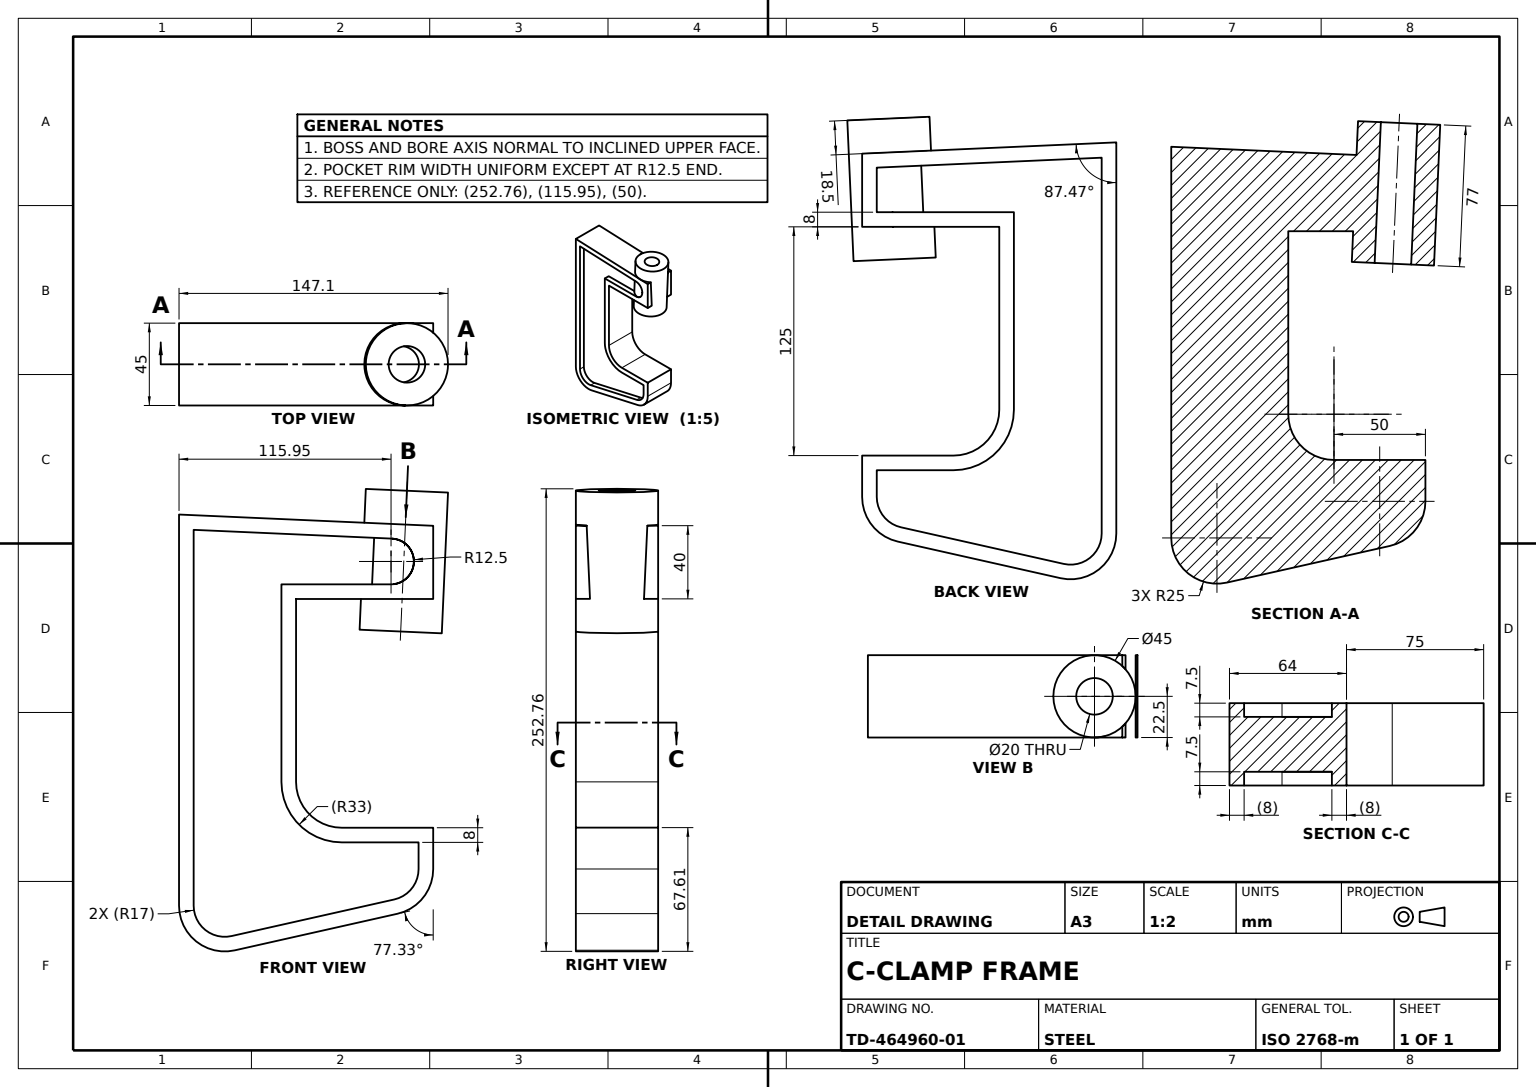
SolidWorks part; units mm, degrees
material "Plain Carbon Steel"
ref_plane "Front Plane" through (0, 0, 0) normal (0, 0, 1) x (1, 0, 0)
ref_plane "Top Plane" through (0, 0, 0) normal (0, 1, 0) x (1, 0, 0)
ref_plane "Right Plane" through (0, 0, 0) normal (1, 0, 0) x (0, 0, -1)
sketch "C Frame Profile Sketch" plane through (0, 0, 0) normal (0, 0, 1) x (1, 0, 0)
  line L0 (108.5187, 232) -> (-30.4813, 238.1503)
  line L1 (-30.4813, 238.1503) -> (-30.4813, 24.3917)
  line L2 (0, 0) -> (89, 20)
  line L7 (33.5187, 92) -> (33.5187, 192)
  line L8 (33.5187, 192) -> (108.5187, 192)
  line L10 (108.5187, 67) -> (108.5187, 44.3917)
  line L11 (58.5187, 67) -> (108.5187, 67)
  line L12 (108.5187, 192) -> (108.5187, 232)
  arc A2 (-30.4813, 24.3917) -> (0, 0) centre (-5.4813, 24.3917) ccw
  arc A3 (108.5187, 44.3917) -> (89, 20) centre (83.5187, 44.3917) cw
  arc A4 (33.5187, 92) -> (58.5187, 67) centre (58.5187, 92) ccw
  point P16 (-30.4813, -6.8497)
  dimension "D1" = 245
  dimension "D3" = 40
  dimension "D4" = 75
  dimension "D5" = 50
  dimension "D6" = 25
  dimension "D8" = 25
  dimension "D2" = 64
  dimension "D7" = 20
  dimension "D9" = 47
  dimension "D10" = 125
extrude "C Frame" add sketch "C Frame Profile Sketch" along normal mid plane 45 contours L12 L0 L1 A2 L2 A3 L10 L11 A4 L7 L8
sketch "Front Pocket Sketch" plane through (0, 0, 22.5) normal (0, 0, 1) x (1, 0, 0)
  line L49 (-22.4813, 229.7885) -> (-22.4813, 24.3917)
  line L50 (100.5187, 224.3461) -> (-22.4813, 229.7885)
  line L51 (100.5187, 200) -> (100.5187, 224.3461)
  line L52 (25.5187, 200) -> (100.5187, 200)
  line L53 (25.5187, 92) -> (25.5187, 200)
  line L54 (100.5187, 59) -> (58.5187, 59)
  line L55 (100.5187, 44.3917) -> (100.5187, 59)
  line L56 (-1.754, 7.8053) -> (87.246, 27.8053)
  line L57 (-22.4813, 229.7885) -> (-22.4813, 24.3917)
  line L58 (86.0173, 224.9878) -> (-22.4813, 229.7885)
  line L60 (25.5187, 200) -> (85.4648, 200)
  line L61 (25.5187, 92) -> (25.5187, 200)
  line L62 (100.5187, 59) -> (58.5187, 59)
  line L63 (100.5187, 44.3917) -> (100.5187, 59)
  line L64 (-1.754, 7.8053) -> (87.246, 27.8053)
  arc A27 (86.0173, 224.9878) -> (85.4648, 200) centre (85.4648, 212.5) cw
  arc A30 (25.5187, 92) -> (58.5187, 59) centre (58.5187, 92) ccw
  arc A31 (87.246, 27.8053) -> (100.5187, 44.3917) centre (83.5187, 44.3917) ccw
  arc A32 (-22.4813, 24.3917) -> (-1.754, 7.8053) centre (-5.4813, 24.3917) ccw
  arc A33 (25.5187, 92) -> (58.5187, 59) centre (58.5187, 92) ccw
  arc A34 (87.246, 27.8053) -> (100.5187, 44.3917) centre (83.5187, 44.3917) ccw
  arc A35 (-22.4813, 24.3917) -> (-1.754, 7.8053) centre (-5.4813, 24.3917) ccw
  dimension "D2" = 12.5
  dimension "D1" = 8
extrude "Front Pocket" cut sketch "Front Pocket Sketch" against normal blind 7.5
sketch "Back Pocket Sketch" plane through (0, 0, -22.5) normal (0, 0, -1) x (-1, 0, 0)
  line L54 (-58.5187, 59) -> (-100.5187, 59)
  line L55 (-25.5187, 200) -> (-25.5187, 92)
  line L56 (-100.5187, 200) -> (-25.5187, 200)
  line L57 (-100.5187, 224.3461) -> (-100.5187, 200)
  line L58 (22.4813, 229.7885) -> (-100.5187, 224.3461)
  line L59 (22.4813, 24.3917) -> (22.4813, 229.7885)
  line L60 (-87.246, 27.8053) -> (1.754, 7.8053)
  line L61 (-100.5187, 59) -> (-100.5187, 44.3917)
  line L62 (-58.5187, 59) -> (-100.5187, 59)
  line L63 (-25.5187, 200) -> (-25.5187, 92)
  line L64 (-100.5187, 200) -> (-25.5187, 200)
  line L65 (-100.5187, 224.3461) -> (-100.5187, 200)
  line L66 (22.4813, 229.7885) -> (-100.5187, 224.3461)
  line L67 (22.4813, 24.3917) -> (22.4813, 229.7885)
  line L68 (-87.246, 27.8053) -> (1.754, 7.8053)
  line L69 (-100.5187, 59) -> (-100.5187, 44.3917)
  arc A23 (-58.5187, 59) -> (-25.5187, 92) centre (-58.5187, 92) ccw
  arc A24 (1.754, 7.8053) -> (22.4813, 24.3917) centre (5.4813, 24.3917) ccw
  arc A25 (-100.5187, 44.3917) -> (-87.246, 27.8053) centre (-83.5187, 44.3917) ccw
  arc A26 (-58.5187, 59) -> (-25.5187, 92) centre (-58.5187, 92) ccw
  arc A27 (1.754, 7.8053) -> (22.4813, 24.3917) centre (5.4813, 24.3917) ccw
  arc A28 (-100.5187, 44.3917) -> (-87.246, 27.8053) centre (-83.5187, 44.3917) ccw
  dimension "D1" = 8
extrude "Back Pocket" cut sketch "Back Pocket Sketch" against normal blind 7.5
sketch "Screw Boss Sketch" plane through (10.4572, 236.3389, 0) normal (0.0442, 0.999, 0) x (0.999, -0.0442, 0)
  line L1 (105.451, -22.5) -> (105.451, 22.5) construction
  line L2 (98.1575, 22.5) -> (-40.9785, 22.5) construction
  line L3 (98.1575, -22.5) -> (-40.9785, -22.5) construction
  circle A0 centre (82.951, 0) radius 22.5
extrude "Screw Boss" add sketch "Screw Boss Sketch" along normal blind 18.5 and the other way blind 58.5
sketch "Screw Hole Sketch" plane through (11.2749, 254.8208, 0) normal (0.0442, 0.999, 0) x (0.999, -0.0442, 0)
  circle A0 centre (82.951, 0) radius 10
  dimension "D1" = 20
extrude "Screw Hole" cut sketch "Screw Hole Sketch" against normal blind 98.5
